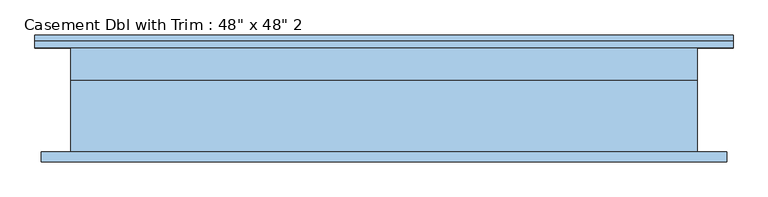
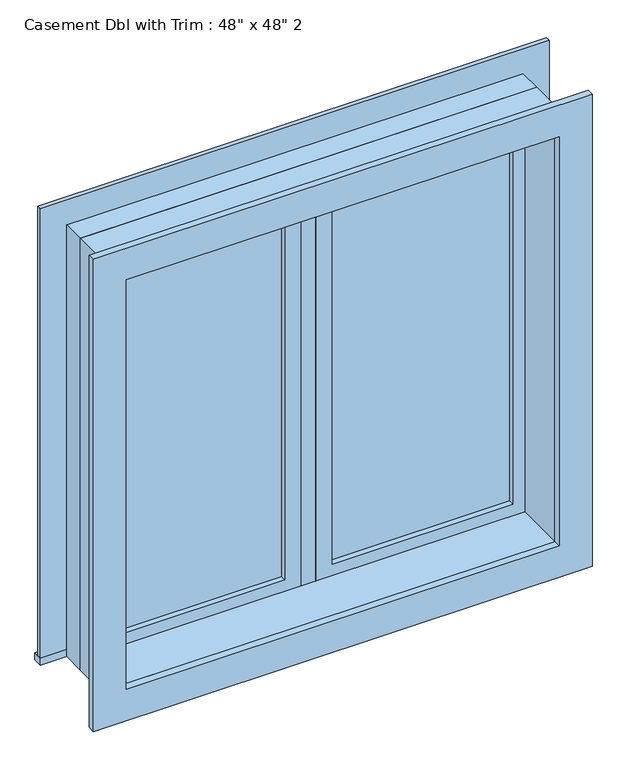
"""IFC4 building model written with IfcOpenShell, lengths in millimetres: window geometry."""

from ifc_helpers import new_model, si_unit, frame, origin, place, context, project, spatial, polyline, outline, extrude, source, transform, mapped, element, save


def window_0862ab64(model_context):
    return source(origin(), model_context, "Body", "SweptSolid", [
        extrude(outline(polyline([(63.5, 85.725), (546.1, 85.725), (546.1, 73.025), (63.5, 73.025), (63.5, 85.725)])), frame((0.0, 0.0, 977.9), z_axis=(0.0, 0.0, 1.0), x_axis=(1.0, 0.0, 0.0)), (0.0, 0.0, 1.0), 1092.2),
        extrude(outline(polyline([(2114.55, 19.05), (933.45, 19.05), (933.45, 590.55), (2114.55, 590.55), (2114.55, 19.05)]), holes=[polyline([(2070.1, 63.5), (2070.1, 546.1), (977.9, 546.1), (977.9, 63.5), (2070.1, 63.5)])]), frame((0.0, 57.15, 0.0), z_axis=(0.0, 1.0, 0.0), x_axis=(0.0, 0.0, 1.0)), (0.0, 0.0, 1.0), 44.45),
        extrude(outline(polyline([(19.05, 57.15), (-19.05, 57.15), (-19.05, 120.65), (19.05, 120.65), (19.05, 57.15)])), frame((0.0, 0.0, 933.45), z_axis=(0.0, 0.0, 1.0), x_axis=(1.0, 0.0, 0.0)), (0.0, 0.0, 1.0), 1181.1),
        extrude(outline(polyline([(-679.45, 146.05), (679.45, 146.05), (679.45, 120.65), (-679.45, 120.65), (-679.45, 146.05)])), frame((0.0, 0.0, 914.4), z_axis=(0.0, 0.0, 1.0), x_axis=(1.0, 0.0, 0.0)), (0.0, 0.0, 1.0), 19.05),
        extrude(outline(polyline([(2114.55, -590.55), (2114.55, 590.55), (933.45, 590.55), (933.45, 679.45), (2203.45, 679.45), (2203.45, -679.45), (933.45, -679.45), (933.45, -590.55), (2114.55, -590.55)])), frame((0.0, 120.65, 0.0), z_axis=(0.0, 1.0, 0.0), x_axis=(0.0, 0.0, 1.0)), (0.0, 0.0, 1.0), 12.7),
        extrude(outline(polyline([(2190.75, 666.75), (2190.75, -666.75), (857.25, -666.75), (857.25, 666.75), (2190.75, 666.75)]), holes=[polyline([(2101.85, 577.85), (946.15, 577.85), (946.15, -577.85), (2101.85, -577.85), (2101.85, 577.85)])]), frame((0.0, -101.6, 0.0), z_axis=(0.0, 1.0, 0.0), x_axis=(0.0, 0.0, 1.0)), (0.0, 0.0, 1.0), 19.05),
        extrude(outline(polyline([(-63.5, 73.025), (-546.1, 73.025), (-546.1, 85.725), (-63.5, 85.725), (-63.5, 73.025)])), frame((0.0, 0.0, 977.9), z_axis=(0.0, 0.0, 1.0), x_axis=(1.0, 0.0, 0.0)), (0.0, 0.0, 1.0), 1092.2),
        extrude(outline(polyline([(2114.55, -590.55), (933.45, -590.55), (933.45, -19.05), (2114.55, -19.05), (2114.55, -590.55)]), holes=[polyline([(2070.1, -546.1), (2070.1, -63.5), (977.9, -63.5), (977.9, -546.1), (2070.1, -546.1)])]), frame((0.0, 57.15, 0.0), z_axis=(0.0, 1.0, 0.0), x_axis=(0.0, 0.0, 1.0)), (0.0, 0.0, 1.0), 44.45),
        extrude(outline(polyline([(2133.6, -609.6), (914.4, -609.6), (914.4, 609.6), (2133.6, 609.6), (2133.6, -609.6)]), holes=[polyline([(2101.85, -577.85), (2101.85, 577.85), (946.15, 577.85), (946.15, -577.85), (2101.85, -577.85)])]), frame((0.0, -82.55, 0.0), z_axis=(0.0, 1.0, 0.0), x_axis=(0.0, 0.0, 1.0)), (0.0, 0.0, 1.0), 139.7),
        extrude(outline(polyline([(2133.6, 609.6), (2133.6, -609.6), (914.4, -609.6), (914.4, 609.6), (2133.6, 609.6)]), holes=[polyline([(2114.55, 590.55), (933.45, 590.55), (933.45, -590.55), (2114.55, -590.55), (2114.55, 590.55)])]), frame((0.0, 57.15, 0.0), z_axis=(0.0, 1.0, 0.0), x_axis=(0.0, 0.0, 1.0)), (0.0, 0.0, 1.0), 63.5),
    ])


if __name__ == "__main__":
    model = new_model("IFC4")
    model_context = context("Model", 3, world=origin())
    ifc_project = project(units=[si_unit("LENGTHUNIT", "METRE", prefix="MILLI")], contexts=[model_context])
    site = spatial("IfcSite", under=ifc_project)
    building = spatial("IfcBuilding", under=site)
    placement = place(None, origin())
    window_shape = window_0862ab64(model_context)
    element("IfcWindow", 1, ObjectType="Casement Dbl with Trim : 48\" x 48\" 2", at=placement, inside=building, context=model_context, shape_type="MappedRepresentation", body=[
        mapped(window_shape, transform((0.0, 0.0, 0.0), x_axis=(1.0, 0.0, 0.0), y_axis=(0.0, 1.0, 0.0), z_axis=(0.0, 0.0, 1.0))),
    ])
    save(model, "model.ifc")

# Revit data of these elements
# Type "Casement Dbl with Trim : 48\" x 48\" 2"
#   Type Mark = "13"
#   Construction Type Id = "GSP4R"
#   Assembly Code = "B2020100"
#   Analytic Construction = "1/8 in Pilkington single glazing"
#   Visual Light Transmittance = 0.9
#   Thermal Resistance (R) = 1.53941 (h·ft²·°F)/BTU
#   Solar Heat Gain Coefficient = 0.78
#   Heat Transfer Coefficient (U) = 0.6496 BTU/(h·ft²·°F)
#   Height = 4' - 0"
#   Default Sill Height = 3' - 0"
#   Trim Projection - Ext. = 0' - 0 1/2"
#   Trim Projection - Int. = 0' - 0 3/4"
#   Trim Width - Exterior = 0' - 3 1/2"
#   Trim Width - Interior = 0' - 3 1/2"
#   Width = 4' - 0"
#   Window Inset = 0' - 0 3/4"
#   Define Thermal Properties by = 1
#   Glass Pane Material = Glass, Clear Glazing
#   Sash Material = Copper
#   Trim Exterior Material = Earth
#   Trim Interior Material = Earth
#   Wall Closure = (empty or 0)
# Element 1 (IfcWindow, "Casement Dbl with Trim : 48\" x 48\" 2")
#   Materials on its faces: "Copper", "Earth", "Glass, Clear Glazing"
# Materials
#   "Glass, Clear Glazing": class "Glass", colour RGB 0 128 192, transparency 0.75, Description = "Clear glazing", Cost = 0
#   "Copper": class "Metal", colour RGB 0 0 0, transparency 0, Description = "Copper, matte finish", Cost = 0
#   "Earth": class "Generic", colour RGB 97 75 62, transparency 0, Description = "Soil", Cost = 0
